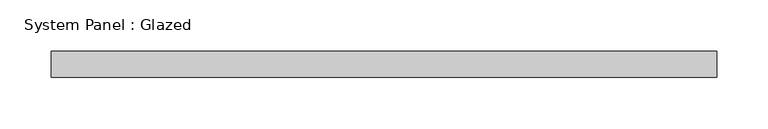
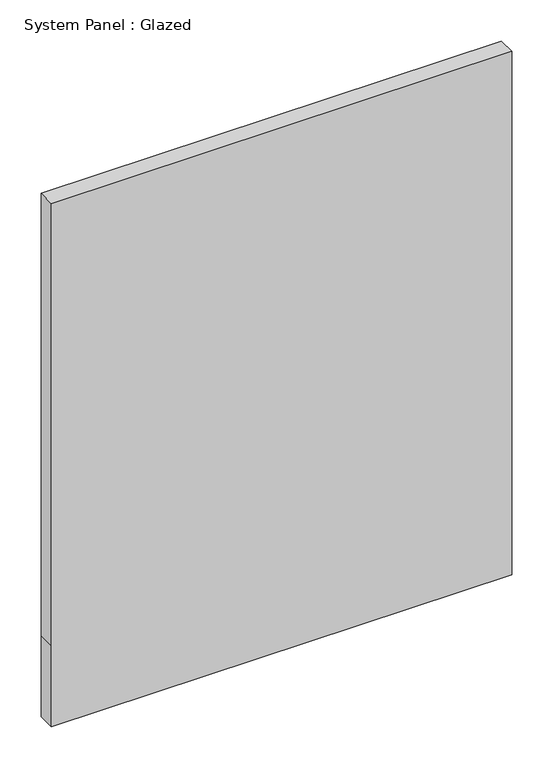
"""IFC4 building model written with IfcOpenShell, lengths in millimetres: plate geometry, System Panel : Glazed."""

from ifc_helpers import new_model, si_unit, frame, origin, place, context, project, spatial, polyline, outline, extrude, source, transform, mapped, element, save


def system_panel_glazed_a09e93fe(model_context):
    return source(origin(), model_context, "Body", "SweptSolid", [
        extrude(outline(polyline([(0.0, -323.85), (0.0, 323.85), (120.65, 323.85), (778.3402035, 323.85), (778.3402035, -323.85), (120.65, -323.85), (0.0, -323.85)])), frame((0.0, 19.05, 0.0), z_axis=(0.0, 1.0, 0.0), x_axis=(0.0, 0.0, 1.0)), (0.0, 0.0, 1.0), 25.4),
    ])


if __name__ == "__main__":
    model = new_model("IFC4")
    model_context = context("Model", 3, world=origin())
    ifc_project = project(units=[si_unit("LENGTHUNIT", "METRE", prefix="MILLI")], contexts=[model_context])
    site = spatial("IfcSite", under=ifc_project)
    building = spatial("IfcBuilding", under=site)
    placement = place(None, origin())
    system_panel_glazed_shape = system_panel_glazed_a09e93fe(model_context)
    element("IfcPlate", 1, ObjectType="System Panel : Glazed", at=placement, inside=building, context=model_context, shape_type="MappedRepresentation", body=[
        mapped(system_panel_glazed_shape, transform((0.0, 0.0, 0.0), x_axis=(1.0, 0.0, 0.0), y_axis=(0.0, 1.0, 0.0), z_axis=(0.0, 0.0, 1.0))),
    ])
    save(model, "model.ifc")

# Revit data of these elements
# Type "System Panel : Glazed"
#   Construction Type Id = "GSP4R"
#   Analytic Construction = "1/8 in Pilkington single glazing"
#   Visual Light Transmittance = 0.9
#   Solar Heat Gain Coefficient = 0.86
#   Heat Transfer Coefficient (U) = 1.18115 BTU/(h·ft²·°F)
#   Define Thermal Properties by = 1
# Element 1 (IfcPlate, "System Panel : Glazed")
#   Materials on its faces: "Glass"
# Materials
#   "Glass": class "Glass", colour RGB 0 128 192, transparency 0.75, Description = "Soda Lime Glass", Cost = 0
